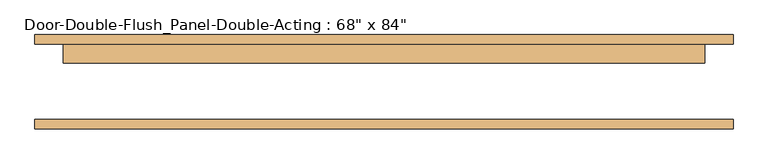
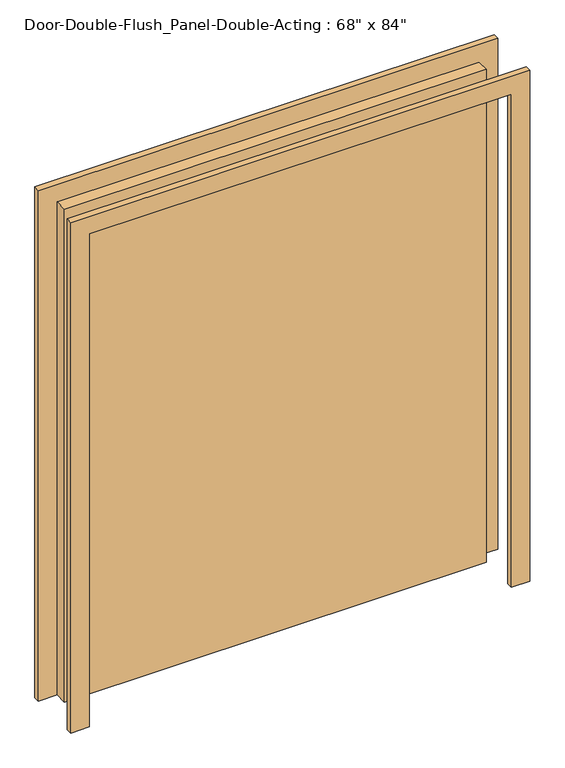
"""IFC4 building model written with IfcOpenShell, lengths in millimetres: door geometry."""

from ifc_helpers import new_model, si_unit, frame, origin, origin_with_axes, place, context, project, spatial, polyline, outline, extrude, source, transform, mapped, element, save


def door_f3de6620(model_context):
    return source(origin(), model_context, "Body", "SweptSolid", [
        extrude(outline(polyline([(2209.8, -939.8), (0.0, -939.8), (0.0, -863.6), (2133.6, -863.6), (2133.6, 863.6), (0.0, 863.6), (0.0, 939.8), (2209.8, 939.8), (2209.8, -939.8)])), frame((0.0, 101.6, 0.0), z_axis=(0.0, 1.0, 0.0), x_axis=(0.0, 0.0, 1.0)), (0.0, 0.0, 1.0), 25.4),
        extrude(outline(polyline([(2133.6, -863.6), (2133.6, 863.6), (0.0, 863.6), (0.0, 939.8), (2209.8, 939.8), (2209.8, -939.8), (0.0, -939.8), (0.0, -863.6), (2133.6, -863.6)])), frame((0.0, -127.0, 0.0), z_axis=(0.0, 1.0, 0.0), x_axis=(0.0, 0.0, 1.0)), (0.0, 0.0, 1.0), 25.4),
        extrude(outline(polyline([(-863.6, 101.6), (863.6, 101.6), (863.6, 50.8), (-863.6, 50.8), (-863.6, 101.6)])), origin_with_axes(), (0.0, 0.0, 1.0), 2133.6),
    ])


if __name__ == "__main__":
    model = new_model("IFC4")
    model_context = context("Model", 3, world=origin())
    ifc_project = project(units=[si_unit("LENGTHUNIT", "METRE", prefix="MILLI")], contexts=[model_context])
    site = spatial("IfcSite", under=ifc_project)
    building = spatial("IfcBuilding", under=site)
    placement = place(None, origin())
    door_shape = door_f3de6620(model_context)
    element("IfcDoor", 1, ObjectType="Door-Double-Flush_Panel-Double-Acting : 68\" x 84\"", at=placement, inside=building, context=model_context, shape_type="MappedRepresentation", body=[
        mapped(door_shape, transform((0.0, 0.0, 0.0), x_axis=(1.0, 0.0, 0.0), y_axis=(0.0, 1.0, 0.0), z_axis=(0.0, 0.0, 1.0))),
    ])
    save(model, "model.ifc")

# Revit data of these elements
# Type "Door-Double-Flush_Panel-Double-Acting : 68\" x 84\""
#   Type Mark = "8"
#   Construction Type Id = "DOOR"
#   Assembly Code = "C1020"
#   Analytic Construction = "Wooden"
#   W = 2' - 10"
#   Thickness = 0' - 2"
#   Thermal Resistance (R) = 2.5876 (h·ft²·°F)/BTU
#   Swing Angle [instance default] = 90.00°
#   Heat Transfer Coefficient (U) = 0.3865 BTU/(h·ft²·°F)
#   Height = 7' - 0"
#   Trim Projection Ext. = 0' - 1"
#   Trim Projection Int. = 0' - 1"
#   Trim Width Ext. = 0' - 3"
#   Trim Width Int. = 0' - 3"
#   Width = 5' - 8"
#   Define Thermal Properties by = 1
#   Panel Material = Wood - Birch - Solid Stained Light Low Gloss
#   Trim Material = Paint - Sienna
#   Visual Light Transmittance = 0
#   Solar Heat Gain Coefficient = 0
#   Function = (empty or 0)
#   Wall Closure = (empty or 0)
# Element 1 (IfcDoor, "Door-Double-Flush_Panel-Double-Acting : 68\" x 84\"")
#   Materials on its faces: "Paint - Sienna", "Wood - Birch - Solid Stained Light Low Gloss"
# Materials
#   "Wood - Birch - Solid Stained Light Low Gloss": class "Wood", colour RGB 210 159 95, transparency 0, Cost = 0
#   "Paint - Sienna": colour RGB 118 70 51, transparency 0, Cost = 0
